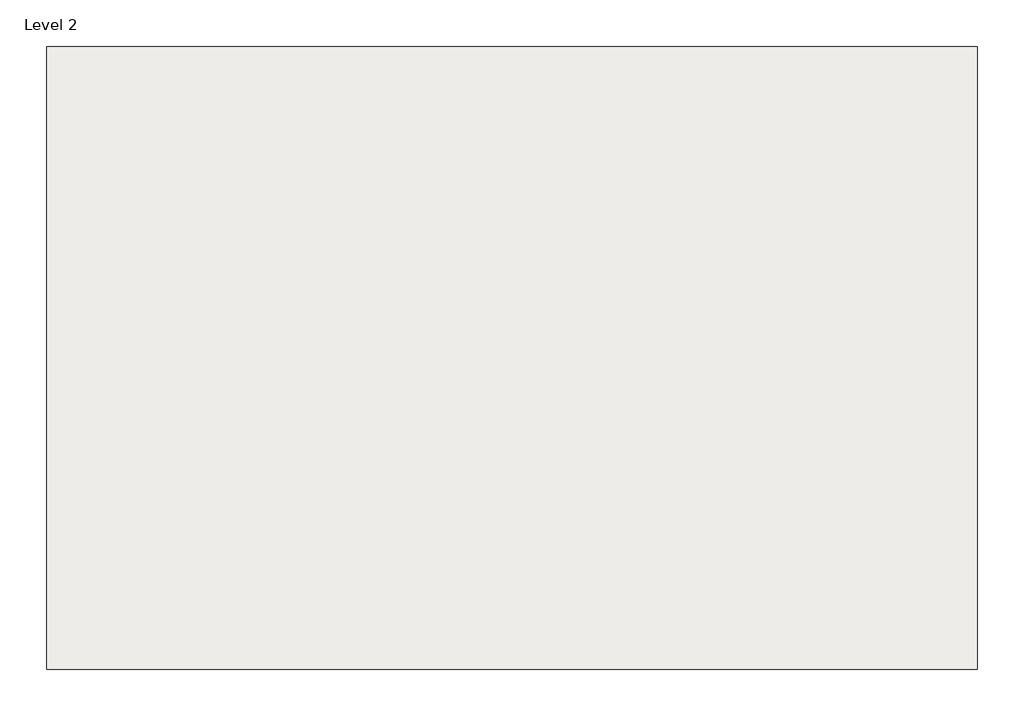
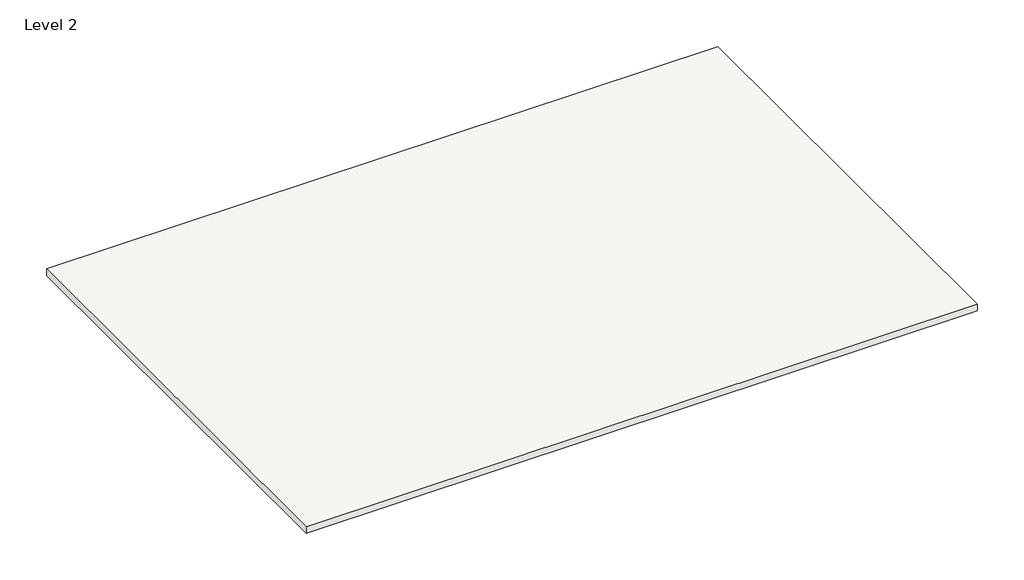
# One storey: 1 roof.
"""IFC4 building model written with IfcOpenShell, lengths in millimetres."""

from ifc_helpers import new_model, si_unit, frame, origin, place, context, project, spatial, polyline, outline, extrude, element, save

model = new_model("IFC4")

# Units and contexts
model_context = context("Model", 3, world=origin())
ifc_project = project(units=[si_unit("LENGTHUNIT", "METRE", prefix="MILLI")], contexts=[model_context])

# Site, building, storey
site = spatial("IfcSite", under=ifc_project)
building = spatial("IfcBuilding", under=site)
storey = spatial("IfcBuildingStorey", under=building, Name="Level 2", Elevation=3048.0)

# Roof
placement = place(None, origin())
element("IfcRoof", 1, ObjectType="Generic - 12\"", at=placement, inside=storey, context=model_context, shape_type="SweptSolid", body=[
    extrude(outline(polyline([(-7944.5640964, 7068.003532), (6625.5109036, 7068.003532), (6625.5109036, -2685.596468), (-7944.5640964, -2685.596468), (-7944.5640964, 7068.003532)])), frame((0.0, 0.0, 3048.0), z_axis=(0.0, 0.0, 1.0), x_axis=(1.0, 0.0, 0.0)), (0.0, 0.0, 1.0), 152.4),
])

save(model, "model.ifc")

# Revit data of these elements
# Type "Generic - 12\""
#   Assembly Code = "B1020"
#   Layers, outside or top first: 0' - 6" no material (function 1)
# Element 1 (IfcRoof, "Generic - 12\"")
#   built-in parameter 1001705 = 10.5 (stored number, unit not read)
#   built-in parameter 1001710 = 33615
#   Phase Created = New Construction
#   Materials on its faces: "Default Roof"
# Materials
#   "Default Roof": colour RGB 88 101 114, transparency 0, Cost = 0
